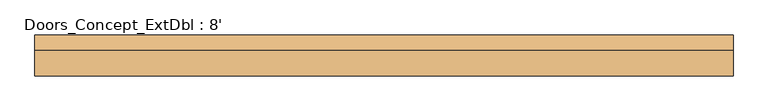
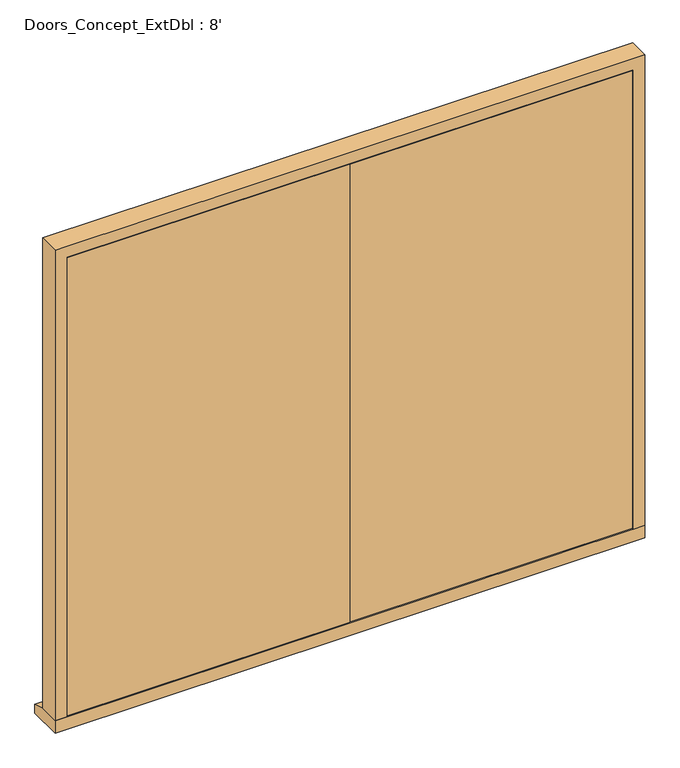
"""IFC4 building model written with IfcOpenShell, lengths in millimetres: door geometry, Doors_Concept_ExtDbl : 8'."""

from ifc_helpers import new_model, si_unit, frame, origin, place, context, project, spatial, polyline, outline, extrude, faceted_brep, source, transform, mapped, element, save


def doors_concept_extdbl_8_449e5563(model_context):
    return source(origin(), model_context, "Body", "SolidModel", [
        faceted_brep([(1148.7, 81.68, 54.5), (1219.2, 81.68, 54.5), (1219.2, -7.32, 54.5), (1170.7, -7.32, 54.5), (1170.7, 39.68, 54.5), (1148.7, 39.68, 54.5), (1148.7, 81.68, 2039.5), (-1148.7, 81.68, 2039.5), (-1148.7, 81.68, 54.5), (-1219.2, 81.68, 54.5), (-1219.2, 81.68, 2110.0), (1219.2, 81.68, 2110.0), (1219.2, -7.32, 2110.0), (-1219.2, -7.32, 2110.0), (-1219.2, -7.32, 54.5), (-1170.7, -7.32, 54.5), (-1170.7, -7.32, 2061.5), (1170.7, -7.32, 2061.5), (1170.7, 39.68, 2061.5), (-1170.7, 39.68, 2061.5), (-1170.7, 39.68, 54.5), (-1148.7, 39.68, 54.5), (-1148.7, 39.68, 2039.5), (1148.7, 39.68, 2039.5)], [[[0, 1, 2, 3, 4, 5]], [[1, 0, 6, 7, 8, 9, 10, 11]], [[2, 1, 11, 12]], [[3, 2, 12, 13, 14, 15, 16, 17]], [[4, 3, 17, 18]], [[5, 4, 18, 19, 20, 21, 22, 23]], [[0, 5, 23, 6]], [[7, 22, 21, 8]], [[8, 21, 20, 15, 14, 9]], [[13, 10, 9, 14]], [[19, 16, 15, 20]], [[12, 11, 10, 13]], [[18, 17, 16, 19]], [[6, 23, 22, 7]]]),
        extrude(outline(polyline([(1167.7, -7.32), (1.5, -7.32), (1.5, 36.68), (1167.7, 36.68), (1167.7, -7.32)])), frame((0.0, 0.0, 58.5), z_axis=(0.0, 0.0, 1.0), x_axis=(1.0, 0.0, 0.0)), (0.0, 0.0, 1.0), 2000.0),
        extrude(outline(polyline([(-1.5, -7.32), (-1167.7, -7.32), (-1167.7, 36.68), (-1.5, 36.68), (-1.5, -7.32)])), frame((0.0, 0.0, 58.5), z_axis=(0.0, 0.0, 1.0), x_axis=(1.0, 0.0, 0.0)), (0.0, 0.0, 1.0), 2000.0),
        extrude(outline(polyline([(-7.32, 0.0), (-7.32, 54.5), (81.68, 54.5), (136.68, 38.5947221), (136.68, 0.0), (-7.32, 0.0)])), frame((-1219.2, 0.0, 0.0), z_axis=(1.0, 0.0, 0.0), x_axis=(0.0, 1.0, 0.0)), (0.0, 0.0, 1.0), 2438.4),
    ])


if __name__ == "__main__":
    model = new_model("IFC4")
    model_context = context("Model", 3, world=origin())
    ifc_project = project(units=[si_unit("LENGTHUNIT", "METRE", prefix="MILLI")], contexts=[model_context])
    site = spatial("IfcSite", under=ifc_project)
    building = spatial("IfcBuilding", under=site)
    placement = place(None, origin())
    doors_concept_extdbl_8_shape = doors_concept_extdbl_8_449e5563(model_context)
    element("IfcDoor", 1, ObjectType="Doors_Concept_ExtDbl : 8'", at=placement, inside=building, context=model_context, shape_type="MappedRepresentation", body=[
        mapped(doors_concept_extdbl_8_shape, transform((0.0, 0.0, 0.0), x_axis=(1.0, 0.0, 0.0), y_axis=(0.0, 1.0, 0.0), z_axis=(0.0, 0.0, 1.0))),
    ])
    save(model, "model.ifc")

# Revit data of these elements
# Type "Doors_Concept_ExtDbl : 8'"
#   Type Mark = "53"
#   Type Comments = "External Double"
#   Operation = "DoubleDoorSingleSwing"
#   Construction Type Id = "GSP4R"
#   Keynote = "L10"
#   Analytic Construction = "1/8 in Pilkington single glazing"
#   Visual Light Transmittance = 0.9
#   Thickness = 0.144357 ft
#   Solar Heat Gain Coefficient = 0.78
#   Rough Width = 8.0 ft
#   Rough Height = 6.922572 ft
#   Heat Transfer Coefficient (U) = 3.6886 W/(m²·K)
#   FrameWidth = 0.137795 ft
#   FrameOffset - External = 0.082021 ft
#   Height = 6.922572 ft
#   Width = 8.0 ft
#   Define Thermal Properties by = 1
#   Function = 1
#   Material Door = Door - Glazing
#   Material Frame = Concept
#   Wall Closure = (empty or 0)
# Element 1 (IfcDoor, "Doors_Concept_ExtDbl : 8'")
#   Materials on its faces: "Concept", "Door - Glazing"
# Materials
#   "Door - Glazing": colour RGB 0 0 255, transparency 0.75
#   "Concept": colour RGB 128 128 255, transparency 0.5
